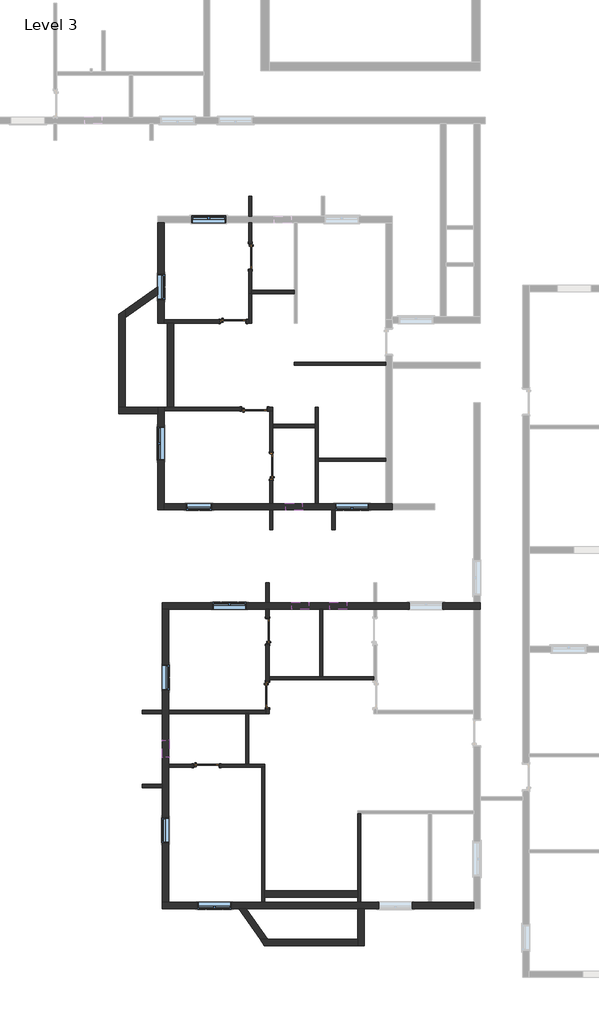
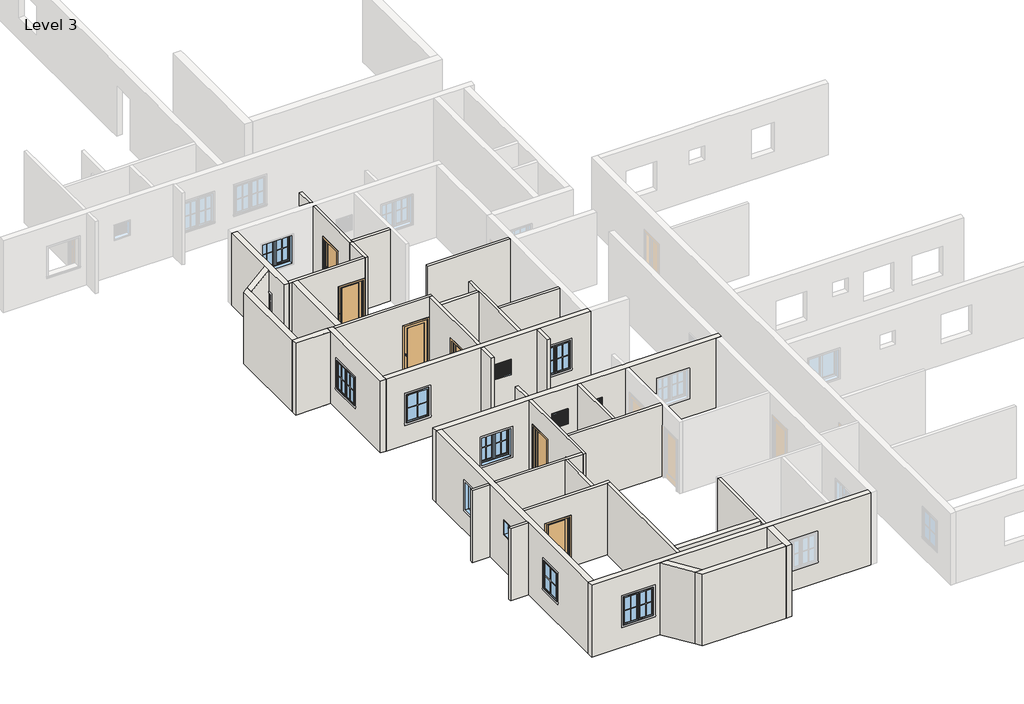
# One storey, part 1 of 7: 39 walls, 13 windows, 7 doors.
# Revit data of these elements (continued)
# Element 51 (IfcWindow, "Window-Casement-Double : 4' x 4'")
#   Mark = "52"
#   Window Inset = 0' - 0"
#   Interior Wall Closure = 0' - 2 1/4"
#   Frame Extension = 0' - 0 1/4"
#   Exterior Wall Closure = 0' - 1 1/4"
#   Interior Trim Visibility = yes
#   Exterior Trim Visibility = yes
#   Phase Created = New Construction
#   Materials on its faces: "Wood - Stained", "Glass", "Clad - White"
# Element 52 (IfcWindow, "Window-Casement-Double : 4' x 4'")
#   Mark = "54"
#   Window Inset = 0' - 0"
#   Interior Wall Closure = 0' - 2 1/4"
#   Frame Extension = 0' - 0 1/4"
#   Exterior Wall Closure = 0' - 1 1/4"
#   Interior Trim Visibility = yes
#   Exterior Trim Visibility = yes
#   Phase Created = New Construction
#   Materials on its faces: "Wood - Stained", "Glass", "Clad - White"
# Element 53 (IfcWindow, "Window-Casement-Double : 4' x 4'")
#   Mark = "56"
#   Window Inset = 0' - 0"
#   Interior Wall Closure = 0' - 2 1/4"
#   Frame Extension = 0' - 0 1/4"
#   Exterior Wall Closure = 0' - 1 1/4"
#   Interior Trim Visibility = yes
#   Exterior Trim Visibility = yes
#   Phase Created = New Construction
#   Materials on its faces: "Wood - Stained", "Glass", "Clad - White"
# Element 54 (IfcWindow, "Window-Casement-Double : 4' x 4'")
#   Mark = "57"
#   Window Inset = 0' - 0"
#   Interior Wall Closure = 0' - 2 1/4"
#   Frame Extension = 0' - 0 1/4"
#   Exterior Wall Closure = 0' - 1 1/4"
#   Interior Trim Visibility = yes
#   Exterior Trim Visibility = yes
#   Phase Created = New Construction
#   Materials on its faces: "Wood - Stained", "Glass", "Clad - White"
# Element 55 (IfcWindow, "Window-Casement-Double : 4' x 4'")
#   Mark = "59"
#   Window Inset = 0' - 0"
#   Interior Wall Closure = 0' - 2 1/4"
#   Frame Extension = 0' - 0 1/4"
#   Exterior Wall Closure = 0' - 1 1/4"
#   Interior Trim Visibility = yes
#   Exterior Trim Visibility = yes
#   Phase Created = New Construction
#   Materials on its faces: "Wood - Stained", "Glass", "Clad - White"
# Element 56 (IfcWindow, "Window-Louvers : 24\" x 24\"")
#   Mark = "8"
#   Blade Width = 1' - 10 1/2"
#   Phase Created = New Construction
#   Materials on its faces: "Birch"
# Element 57 (IfcWindow, "Window-Louvers : 24\" x 24\"")
#   Mark = "11"
#   Blade Width = 1' - 10 1/2"
#   Phase Created = New Construction
#   Materials on its faces: "Birch"
# Element 58 (IfcWindow, "Window-Louvers : 24\" x 24\"")
#   Mark = "12"
#   Blade Width = 1' - 10 1/2"
#   Phase Created = New Construction
#   Materials on its faces: "Birch"
# Element 59 (IfcWindow, "Window-Louvers : 24\" x 24\"")
#   Mark = "14"
#   Blade Width = 1' - 10 1/2"
#   Phase Created = New Construction
#   Materials on its faces: "Birch"
# Materials
#   "Cherry": class "Wood", colour RGB 226 177 128, transparency 0, Description = "Prunus Serotina", Cost = 0
#   "Aluminum": class "Metal", colour RGB 247 247 247, transparency 0, Description = "Aluminum 6061", Cost = 0
#   "Wood - Stained": class "Wood", colour RGB 224 178 126, transparency 0, Cost = 0
#   "Glass": class "Glass", colour RGB 0 128 192, transparency 0.75, Description = "Soda Lime Glass", Cost = 0
#   "Clad - White": class "Wood", colour RGB 242 242 238, transparency 0, Cost = 0
#   "Birch": class "Wood", colour RGB 224 178 126, transparency 0, Description = "Betula Alleghaniensis", Cost = 0
#   "Default Wall": colour RGB 128 128 128, transparency 0, Cost = 0
